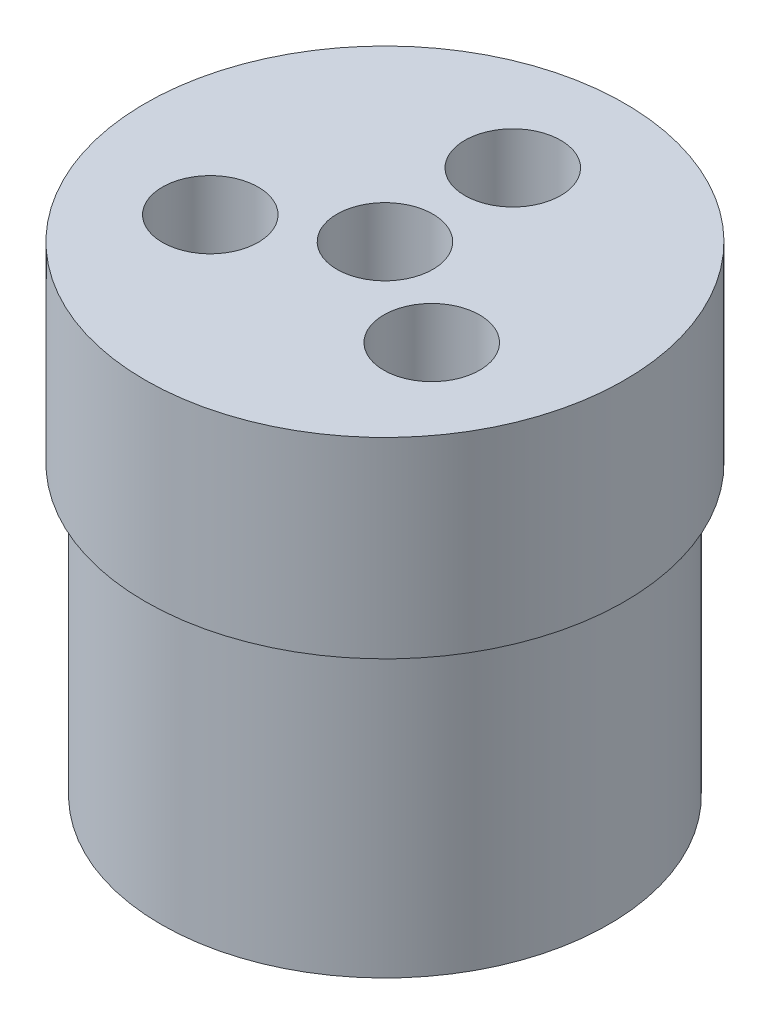
ISO-10303-21;
HEADER;
FILE_DESCRIPTION(('STEP AP214'),'2;1');
FILE_NAME('part.step','',(''),(''),'','','');
FILE_SCHEMA(('AUTOMOTIVE_DESIGN { 1 0 10303 214 1 1 1 1 }'));
ENDSEC;
DATA;
#1=APPLICATION_CONTEXT('core data for automotive mechanical design processes');
#2=APPLICATION_PROTOCOL_DEFINITION('international standard','automotive_design',2000,#1);
#3=PRODUCT_CONTEXT('',#1,'mechanical');
#4=PRODUCT('Part','Part','',(#3));
#5=PRODUCT_RELATED_PRODUCT_CATEGORY('part','',(#4));
#6=PRODUCT_DEFINITION_FORMATION('','',#4);
#7=PRODUCT_DEFINITION_CONTEXT('part definition',#1,'design');
#8=PRODUCT_DEFINITION('design','',#6,#7);
#9=PRODUCT_DEFINITION_SHAPE('','',#8);
#10=(LENGTH_UNIT() NAMED_UNIT(*) SI_UNIT(.MILLI.,.METRE.));
#11=(NAMED_UNIT(*) PLANE_ANGLE_UNIT() SI_UNIT($,.RADIAN.));
#12=(NAMED_UNIT(*) SI_UNIT($,.STERADIAN.) SOLID_ANGLE_UNIT());
#13=UNCERTAINTY_MEASURE_WITH_UNIT(LENGTH_MEASURE(1.E-05),#10,'distance_accuracy_value','');
#14=(GEOMETRIC_REPRESENTATION_CONTEXT(3) GLOBAL_UNCERTAINTY_ASSIGNED_CONTEXT((#13)) GLOBAL_UNIT_ASSIGNED_CONTEXT((#10,
#11,#12)) REPRESENTATION_CONTEXT('',''));
#15=CARTESIAN_POINT('',(0.,0.,0.));
#16=DIRECTION('',(0.,0.,1.));
#17=DIRECTION('',(1.,0.,0.));
#18=AXIS2_PLACEMENT_3D('',#15,#16,#17);
#19=CARTESIAN_POINT('',(0.,12.,0.));
#20=DIRECTION('',(0.,-1.,0.));
#21=DIRECTION('',(0.,0.,-1.));
#22=AXIS2_PLACEMENT_3D('',#19,#20,#21);
#23=CYLINDRICAL_SURFACE('',#22,15.);
#24=CARTESIAN_POINT('',(0.,12.,0.));
#25=DIRECTION('',(0.,1.,0.));
#26=DIRECTION('',(0.,0.,1.));
#27=AXIS2_PLACEMENT_3D('',#24,#25,#26);
#28=CIRCLE('',#27,15.);
#29=CARTESIAN_POINT('',(0.,12.,15.));
#30=VERTEX_POINT('',#29);
#31=EDGE_CURVE('E42',#30,#30,#28,.T.);
#32=ORIENTED_EDGE('',*,*,#31,.F.);
#33=EDGE_LOOP('',(#32));
#34=FACE_BOUND('',#33,.T.);
#35=CARTESIAN_POINT('',(0.,0.,0.));
#36=DIRECTION('',(0.,1.,0.));
#37=DIRECTION('',(0.,0.,1.));
#38=AXIS2_PLACEMENT_3D('',#35,#36,#37);
#39=CIRCLE('',#38,15.);
#40=CARTESIAN_POINT('',(0.,0.,15.));
#41=VERTEX_POINT('',#40);
#42=EDGE_CURVE('E47',#41,#41,#39,.T.);
#43=ORIENTED_EDGE('',*,*,#42,.T.);
#44=EDGE_LOOP('',(#43));
#45=FACE_BOUND('',#44,.T.);
#46=ADVANCED_FACE('F40',(#34,#45),#23,.T.);
#47=CARTESIAN_POINT('',(0.,12.,0.));
#48=DIRECTION('',(0.,1.,0.));
#49=DIRECTION('',(0.,0.,1.));
#50=AXIS2_PLACEMENT_3D('',#47,#48,#49);
#51=PLANE('',#50);
#52=CARTESIAN_POINT('',(0.,12.,0.));
#53=DIRECTION('',(0.,1.,0.));
#54=DIRECTION('',(0.,0.,1.));
#55=AXIS2_PLACEMENT_3D('',#52,#53,#54);
#56=CIRCLE('',#55,3.);
#57=CARTESIAN_POINT('',(0.,12.,3.));
#58=VERTEX_POINT('',#57);
#59=EDGE_CURVE('E102',#58,#58,#56,.T.);
#60=ORIENTED_EDGE('',*,*,#59,.F.);
#61=EDGE_LOOP('',(#60));
#62=FACE_BOUND('',#61,.T.);
#63=CARTESIAN_POINT('',(0.,12.,-8.));
#64=DIRECTION('',(0.,1.,0.));
#65=DIRECTION('',(0.,0.,1.));
#66=AXIS2_PLACEMENT_3D('',#63,#64,#65);
#67=CIRCLE('',#66,3.);
#68=CARTESIAN_POINT('',(0.,12.,-5.));
#69=VERTEX_POINT('',#68);
#70=EDGE_CURVE('E63',#69,#69,#67,.T.);
#71=ORIENTED_EDGE('',*,*,#70,.F.);
#72=EDGE_LOOP('',(#71));
#73=FACE_BOUND('',#72,.T.);
#74=CARTESIAN_POINT('',(6.92820323027602,12.,3.99999999999971));
#75=DIRECTION('',(0.,1.,0.));
#76=DIRECTION('',(0.,0.,1.));
#77=AXIS2_PLACEMENT_3D('',#74,#75,#76);
#78=CIRCLE('',#77,3.00000000000044);
#79=CARTESIAN_POINT('',(6.92820323027602,12.,7.00000000000014));
#80=VERTEX_POINT('',#79);
#81=EDGE_CURVE('E112',#80,#80,#78,.T.);
#82=ORIENTED_EDGE('',*,*,#81,.F.);
#83=EDGE_LOOP('',(#82));
#84=FACE_BOUND('',#83,.T.);
#85=CARTESIAN_POINT('',(-6.928203230275,12.,4.0000000000003));
#86=DIRECTION('',(0.,1.,0.));
#87=DIRECTION('',(0.,0.,1.));
#88=AXIS2_PLACEMENT_3D('',#85,#86,#87);
#89=CIRCLE('',#88,3.00000000000065);
#90=CARTESIAN_POINT('',(-6.928203230275,12.,7.00000000000095));
#91=VERTEX_POINT('',#90);
#92=EDGE_CURVE('E111',#91,#91,#89,.T.);
#93=ORIENTED_EDGE('',*,*,#92,.F.);
#94=EDGE_LOOP('',(#93));
#95=FACE_BOUND('',#94,.T.);
#96=ORIENTED_EDGE('',*,*,#31,.T.);
#97=EDGE_LOOP('',(#96));
#98=FACE_BOUND('',#97,.T.);
#99=ADVANCED_FACE('F81',(#62,#73,#84,#95,#98),#51,.T.);
#100=CARTESIAN_POINT('',(0.,0.,0.));
#101=DIRECTION('',(0.,1.,0.));
#102=DIRECTION('',(0.,0.,1.));
#103=AXIS2_PLACEMENT_3D('',#100,#101,#102);
#104=PLANE('',#103);
#105=CARTESIAN_POINT('',(0.,0.,0.));
#106=DIRECTION('',(0.,-1.,0.));
#107=DIRECTION('',(0.,0.,-1.));
#108=AXIS2_PLACEMENT_3D('',#105,#106,#107);
#109=CIRCLE('',#108,14.);
#110=CARTESIAN_POINT('',(0.,0.,-14.));
#111=VERTEX_POINT('',#110);
#112=EDGE_CURVE('E10',#111,#111,#109,.T.);
#113=ORIENTED_EDGE('',*,*,#112,.F.);
#114=EDGE_LOOP('',(#113));
#115=FACE_BOUND('',#114,.T.);
#116=ORIENTED_EDGE('',*,*,#42,.F.);
#117=EDGE_LOOP('',(#116));
#118=FACE_BOUND('',#117,.T.);
#119=ADVANCED_FACE('F74',(#115,#118),#104,.F.);
#120=CARTESIAN_POINT('',(0.,-18.,0.));
#121=DIRECTION('',(0.,1.,0.));
#122=DIRECTION('',(0.,0.,1.));
#123=AXIS2_PLACEMENT_3D('',#120,#121,#122);
#124=CYLINDRICAL_SURFACE('',#123,14.);
#125=CARTESIAN_POINT('',(0.,-18.,0.));
#126=DIRECTION('',(0.,-1.,0.));
#127=DIRECTION('',(0.,0.,-1.));
#128=AXIS2_PLACEMENT_3D('',#125,#126,#127);
#129=CIRCLE('',#128,14.);
#130=CARTESIAN_POINT('',(0.,-18.,-14.));
#131=VERTEX_POINT('',#130);
#132=EDGE_CURVE('E55',#131,#131,#129,.T.);
#133=ORIENTED_EDGE('',*,*,#132,.F.);
#134=EDGE_LOOP('',(#133));
#135=FACE_BOUND('',#134,.T.);
#136=ORIENTED_EDGE('',*,*,#112,.T.);
#137=EDGE_LOOP('',(#136));
#138=FACE_BOUND('',#137,.T.);
#139=ADVANCED_FACE('F75',(#135,#138),#124,.T.);
#140=CARTESIAN_POINT('',(0.,-18.,0.));
#141=DIRECTION('',(0.,-1.,0.));
#142=DIRECTION('',(0.,0.,-1.));
#143=AXIS2_PLACEMENT_3D('',#140,#141,#142);
#144=PLANE('',#143);
#145=CARTESIAN_POINT('',(0.,-18.,0.));
#146=DIRECTION('',(0.,-1.,0.));
#147=DIRECTION('',(0.,0.,-1.));
#148=AXIS2_PLACEMENT_3D('',#145,#146,#147);
#149=CIRCLE('',#148,3.);
#150=CARTESIAN_POINT('',(0.,-18.,-3.));
#151=VERTEX_POINT('',#150);
#152=EDGE_CURVE('E37',#151,#151,#149,.T.);
#153=ORIENTED_EDGE('',*,*,#152,.F.);
#154=EDGE_LOOP('',(#153));
#155=FACE_BOUND('',#154,.T.);
#156=CARTESIAN_POINT('',(0.,-18.,-8.));
#157=DIRECTION('',(0.,-1.,0.));
#158=DIRECTION('',(0.,0.,-1.));
#159=AXIS2_PLACEMENT_3D('',#156,#157,#158);
#160=CIRCLE('',#159,3.);
#161=CARTESIAN_POINT('',(0.,-18.,-11.));
#162=VERTEX_POINT('',#161);
#163=EDGE_CURVE('E62',#162,#162,#160,.T.);
#164=ORIENTED_EDGE('',*,*,#163,.F.);
#165=EDGE_LOOP('',(#164));
#166=FACE_BOUND('',#165,.T.);
#167=CARTESIAN_POINT('',(6.92820323027602,-18.,3.99999999999971));
#168=DIRECTION('',(0.,-1.,0.));
#169=DIRECTION('',(0.,0.,-1.));
#170=AXIS2_PLACEMENT_3D('',#167,#168,#169);
#171=CIRCLE('',#170,3.00000000000044);
#172=CARTESIAN_POINT('',(6.92820323027602,-18.,0.999999999999266));
#173=VERTEX_POINT('',#172);
#174=EDGE_CURVE('E58',#173,#173,#171,.T.);
#175=ORIENTED_EDGE('',*,*,#174,.F.);
#176=EDGE_LOOP('',(#175));
#177=FACE_BOUND('',#176,.T.);
#178=CARTESIAN_POINT('',(-6.928203230275,-18.,4.0000000000003));
#179=DIRECTION('',(0.,-1.,0.));
#180=DIRECTION('',(0.,0.,-1.));
#181=AXIS2_PLACEMENT_3D('',#178,#179,#180);
#182=CIRCLE('',#181,3.00000000000065);
#183=CARTESIAN_POINT('',(-6.928203230275,-18.,0.999999999999651));
#184=VERTEX_POINT('',#183);
#185=EDGE_CURVE('E60',#184,#184,#182,.T.);
#186=ORIENTED_EDGE('',*,*,#185,.F.);
#187=EDGE_LOOP('',(#186));
#188=FACE_BOUND('',#187,.T.);
#189=ORIENTED_EDGE('',*,*,#132,.T.);
#190=EDGE_LOOP('',(#189));
#191=FACE_BOUND('',#190,.T.);
#192=ADVANCED_FACE('F68',(#155,#166,#177,#188,#191),#144,.T.);
#193=CARTESIAN_POINT('',(-6.928203230275,-32.,4.0000000000003));
#194=DIRECTION('',(0.,1.,0.));
#195=DIRECTION('',(0.,0.,1.));
#196=AXIS2_PLACEMENT_3D('',#193,#194,#195);
#197=CYLINDRICAL_SURFACE('',#196,3.00000000000065);
#198=ORIENTED_EDGE('',*,*,#185,.T.);
#199=EDGE_LOOP('',(#198));
#200=FACE_BOUND('',#199,.T.);
#201=ORIENTED_EDGE('',*,*,#92,.T.);
#202=EDGE_LOOP('',(#201));
#203=FACE_BOUND('',#202,.T.);
#204=ADVANCED_FACE('F82',(#200,#203),#197,.F.);
#205=CARTESIAN_POINT('',(6.92820323027602,-32.,3.99999999999971));
#206=DIRECTION('',(0.,1.,0.));
#207=DIRECTION('',(0.,0.,1.));
#208=AXIS2_PLACEMENT_3D('',#205,#206,#207);
#209=CYLINDRICAL_SURFACE('',#208,3.00000000000044);
#210=ORIENTED_EDGE('',*,*,#174,.T.);
#211=EDGE_LOOP('',(#210));
#212=FACE_BOUND('',#211,.T.);
#213=ORIENTED_EDGE('',*,*,#81,.T.);
#214=EDGE_LOOP('',(#213));
#215=FACE_BOUND('',#214,.T.);
#216=ADVANCED_FACE('F126',(#212,#215),#209,.F.);
#217=CARTESIAN_POINT('',(0.,-32.,-8.));
#218=DIRECTION('',(0.,1.,0.));
#219=DIRECTION('',(0.,0.,1.));
#220=AXIS2_PLACEMENT_3D('',#217,#218,#219);
#221=CYLINDRICAL_SURFACE('',#220,3.);
#222=ORIENTED_EDGE('',*,*,#163,.T.);
#223=EDGE_LOOP('',(#222));
#224=FACE_BOUND('',#223,.T.);
#225=ORIENTED_EDGE('',*,*,#70,.T.);
#226=EDGE_LOOP('',(#225));
#227=FACE_BOUND('',#226,.T.);
#228=ADVANCED_FACE('F125',(#224,#227),#221,.F.);
#229=CARTESIAN_POINT('',(0.,-32.,0.));
#230=DIRECTION('',(0.,1.,0.));
#231=DIRECTION('',(0.,0.,1.));
#232=AXIS2_PLACEMENT_3D('',#229,#230,#231);
#233=CYLINDRICAL_SURFACE('',#232,3.);
#234=ORIENTED_EDGE('',*,*,#152,.T.);
#235=EDGE_LOOP('',(#234));
#236=FACE_BOUND('',#235,.T.);
#237=ORIENTED_EDGE('',*,*,#59,.T.);
#238=EDGE_LOOP('',(#237));
#239=FACE_BOUND('',#238,.T.);
#240=ADVANCED_FACE('F122',(#236,#239),#233,.F.);
#241=CLOSED_SHELL('',(#46,#99,#119,#139,#192,#204,#216,#228,#240));
#242=MANIFOLD_SOLID_BREP('B2',#241);
#243=ADVANCED_BREP_SHAPE_REPRESENTATION('',(#18,#242),#14);
#244=SHAPE_DEFINITION_REPRESENTATION(#9,#243);
ENDSEC;
END-ISO-10303-21;
